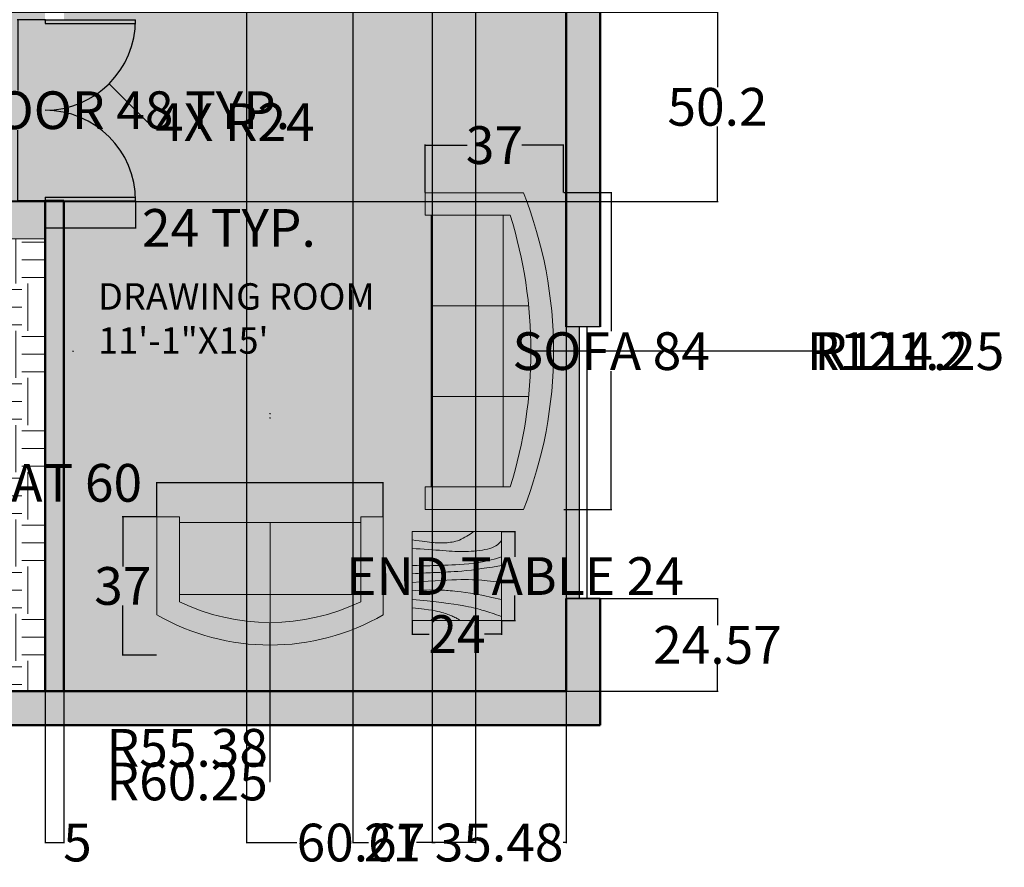
# Model space of a CAD drawing. Units: inches. Extents: x 77 to 548, y 631 to 1307.
# Tile 2 of 4: x 287 to 548, y 631 to 856. Entities that reach past the tile are written whole.
import ezdxf

# ---------------------------------------------------------------- set-up
doc = ezdxf.new("R2010")
doc.units = ezdxf.units.IN
doc.header["$MEASUREMENT"] = 0
for name, color, linetype, lineweight in [('A-ANNO-DIMS', 2, 'Continuous', 18), ('A-AREA-IDEN', 7, 'Continuous', 18), ('A-FLOR-STRS', 7, 'Continuous', 25), ('A-WALL', 7, 'Continuous', 50), ('DOORS', 4, 'Continuous', 25), ('FURNITURE', 34, 'Continuous', 18), ('WINDOW', 6, 'Continuous', 25)]:
    doc.layers.add(name, color=color, linetype=linetype, lineweight=lineweight)
for name, color, linetype, lineweight, true_color in [('A-FLOR-PATT', 254, 'Continuous', 13, 0xd7ebd2), ('A-WALL-PATT', 252, 'Continuous', 13, 0x939598), ('C-PVMT-PATT', 31, 'Continuous', 13, 0xfecc66)]:
    doc.layers.add(name, color=color, linetype=linetype, lineweight=lineweight, true_color=true_color)
doc.styles.get("Standard").update_dxf_attribs({"font": 'arial.ttf'})
doc.dimstyles.get("Standard").update_dxf_attribs({"dimtxt": 10, "dimasz": 0.18, "dimexe": 0.18, "dimexo": 0.0625, "dimgap": 0.09, "dimtad": 0, "dimtih": 1, "dimtoh": 1, "dimdec": 0, "dimzin": 0, "dimdsep": 46, "dimlunit": 3, "dimtxsty": 'Standard', "dimcen": 0.09, "dimadec": 0, "dimazin": 0, "dimtfac": 1, "dimtdec": 0, "dimtofl": 0, "dimtmove": 0, "dimatfit": 3, "dimfxl": 1, "dimtolj": 1, "dimtzin": 0, "dimarcsym": 0})

# ---------------------------------------------------------------- blocks, each defined once
blk = doc.blocks.new('Table - Square Woodgrain 42 x 42 in.')
blk.add_line((0, -42), (42, -42))
for points in [[(0, -4), (1.704, -4.2172), (3.2358, -4.4188), (4.615, -4.604), (5.8615, -4.7721), (6.9951, -4.9224), (8.0357, -5.0541), (9.0031, -5.1667), (9.9171, -5.2594), (10.7951, -5.3316), (11.6445, -5.3836), (12.4702, -5.4157), (13.277, -5.4283), (14.0698, -5.4217), (14.8535, -5.3964), (15.6331, -5.3526), (16.4133, -5.2908), (17.1986, -5.2103), (17.9913, -5.1062), (18.793, -4.9727), (19.6056, -4.8038), (20.4307, -4.5937), (21.2701, -4.3365), (22.1256, -4.0262), (22.9989, -3.6571), (23.888, -3.2272), (24.7756, -2.7516), (25.6408, -2.2491), (26.4624, -1.7387), (27.2195, -1.2395), (27.891, -0.7703), (28.456, -0.3501), (28.8934, 0.002)], [(0, -42), (0, 0), (42, 0), (42, -42)], [(0, -8), (1.8203, -8.1001), (3.6741, -8.2149), (5.5411, -8.3408), (7.4011, -8.4741), (9.2339, -8.6112), (11.0193, -8.7484), (12.7371, -8.8821), (14.3671, -9.0086), (15.8954, -9.1246), (17.3337, -9.2278), (18.6997, -9.3159), (20.0116, -9.387), (21.2871, -9.4389), (22.5442, -9.4696), (23.8008, -9.477), (25.0749, -9.459), (26.3791, -9.4137), (27.7049, -9.3403), (29.0383, -9.2382), (30.3655, -9.1068), (31.6728, -8.9455), (32.9461, -8.7535), (34.1717, -8.5304), (35.3358, -8.2756), (36.4268, -7.9863), (37.443, -7.6521), (38.3849, -7.2603), (39.253, -6.7986), (40.048, -6.2542), (40.7705, -5.6147), (41.421, -4.8674), (42, -4)], [(42, -12), (39.1784, -12.8621), (36.4519, -13.5654), (33.8246, -14.1294), (31.3004, -14.5731), (28.8832, -14.9161), (26.577, -15.1775), (24.3858, -15.3768), (22.3136, -15.5332), (20.3622, -15.6632), (18.5254, -15.7718), (16.7947, -15.8612), (15.1618, -15.9338), (13.6183, -15.9916), (12.1558, -16.0369), (10.7659, -16.0718), (9.4403, -16.0987), (8.1703, -16.1191), (6.9461, -16.1325), (5.7577, -16.1377), (4.595, -16.1335), (3.4479, -16.1188), (2.3064, -16.0924), (1.1604, -16.0532), (0, -16)], [(42, -16), (37.6529, -16.7365), (33.8802, -17.329), (30.6179, -17.7961), (27.8015, -18.1561), (25.3668, -18.4275), (23.2497, -18.6288), (21.3859, -18.7785), (19.7111, -18.8949), (18.1693, -18.9939), (16.7375, -19.0795), (15.401, -19.1534), (14.1449, -19.217), (12.9544, -19.2717), (11.8148, -19.3191), (10.7113, -19.3606), (9.6291, -19.3976), (8.5534, -19.4323), (7.47, -19.4689), (6.3643, -19.5122), (5.222, -19.5672), (4.0288, -19.6386), (2.7703, -19.7313), (1.4321, -19.8501), (0, -20)], [(0, -24), (3.9243, -23.6805), (7.4766, -23.4138), (10.6891, -23.1954), (13.5943, -23.0205), (16.2247, -22.8847), (18.6125, -22.7832), (20.7903, -22.7116), (22.7903, -22.6651), (24.6563, -22.642), (26.4764, -22.6507), (28.35, -22.7024), (30.3766, -22.8084), (32.6555, -22.98), (35.2861, -23.2283), (38.3678, -23.5645), (42, -24)], [(42, -32), (37.392, -31.017), (33.4585, -30.2231), (30.1291, -29.5949), (27.3334, -29.109), (25.0009, -28.742), (23.0612, -28.4707), (21.4439, -28.2716), (20.0786, -28.1215), (18.8998, -28.0002), (17.8609, -27.9014), (16.9206, -27.8219), (16.0371, -27.7588), (15.1691, -27.709), (14.2748, -27.6693), (13.3128, -27.6368), (12.2415, -27.6083), (11.0295, -27.5824), (9.6867, -27.5643), (8.233, -27.5608), (6.6884, -27.5787), (5.0728, -27.6248), (3.4062, -27.7058), (1.7086, -27.8286), (0, -28)], [(0, -32), (5.4026, -32.5358), (9.9494, -33.019), (13.7424, -33.4553), (16.8834, -33.8505), (19.4743, -34.2106), (21.6171, -34.5413), (23.4136, -34.8486), (24.9657, -35.1382), (26.3614, -35.4156), (27.6332, -35.6841), (28.7995, -35.9467), (29.8788, -36.2064), (30.8897, -36.4661), (31.8507, -36.7288), (32.7802, -36.9973), (33.6968, -37.2747), (34.6175, -37.5635), (35.5531, -37.8651), (36.5128, -38.1805), (37.506, -38.5108), (38.5421, -38.8568), (39.6302, -39.2197), (40.7797, -39.6004), (42, -40)], [(0, -36), (3.0098, -36.2857), (5.5354, -36.5643), (7.6368, -36.8359), (9.374, -37.1009), (10.807, -37.3597), (11.9957, -37.6126), (13.0002, -37.8599), (13.8804, -38.102), (14.6874, -38.3393), (15.4365, -38.5729), (16.1338, -38.8041), (16.7858, -39.0341), (17.3987, -39.264), (17.9787, -39.4952), (18.5322, -39.7288), (19.0655, -39.9662), (19.5832, -40.2081), (20.0842, -40.4544), (20.5657, -40.7046), (21.0249, -40.9581), (21.459, -41.2144), (21.8653, -41.4731), (22.2409, -41.7335), (22.5831, -41.9951)]]:
    blk.add_lwpolyline(points)
blk = doc.blocks.new('Sofa - Roundback 7 ft.')
for p, q in [((-12.00002, -32.4421), (-12.00003, -6.5971)), ((11.99997, -32.4421), (11.99998, -6.5971)), ((-36.000027, -34), (-36.000027, -11.4696)), ((35.99998, -34), (35.99998, -11.4696)), ((-35.999844, -13.3819), (35.9998, -13.3819)), ((-36.000027, -32.4421), (35.99998, -32.4421))]:
    blk.add_line(p, q)
for points in [[(-36.000027, -34), (-42.000027, -34), (-42.000027, -8)], [(41.99998, -8), (41.99998, -34), (35.99998, -34)]]:
    blk.add_lwpolyline(points)
for centre, radius, start, end in [((0, -114.25), 114.25, 68.43141, 111.5686), ((-0.00001, -127.1968), 121.1968, 72.72033, 107.2797)]:
    blk.add_arc(centre, radius, start, end)
blk = doc.blocks.new('Sofa - Roundback Loveseat 5 ft.')
for p, q in [((0, -32.44198), (0, -5.99998)), ((-24, -33.99998), (-24, -11.46958)), ((24.00004, -33.99998), (24.00004, -11.46958)), ((-23.9998, -13.38178), (23.99986, -13.38178)), ((-24, -32.44198), (24.00004, -32.44198))]:
    blk.add_line(p, q)
for points in [[(-24, -33.99998), (-30, -33.99998), (-30, -7.99998)], [(30.00004, -7.99998), (30.00004, -33.99998), (24.00004, -33.99998)]]:
    blk.add_lwpolyline(points)
for centre, radius, start, end in [((0, -60.24998), 60.24998, 60.13715, 119.8628), ((0, -61.38438), 55.38444, 64.32083, 115.6792)]:
    blk.add_arc(centre, radius, start, end)
blk = doc.blocks.new('WINDOW-72')
for p, q in [((9, 72), (0, 72)), ((3.5, 72), (3.5, 0)), ((5.5, 72), (5.5, 0)), ((9, 0), (0, 0))]:
    blk.add_line(p, q)
blk = doc.blocks.new('DOOR-DOUBLE-48')
for p, q in [((0, 0), (0, 24)), ((1, 0), (1, 23.98)), ((47, 0), (47, 23.98)), ((48, 0), (48, 24)), ((0, 0), (1, 0)), ((47, 0), (48, 0))]:
    blk.add_line(p, q)
for centre, start, end in [((0, 0), 0, 90), ((48, 0), 90, 180)]:
    blk.add_arc(centre, 24, start, end)
blk = doc.blocks.new('*D26')
at = {"layer": 'A-ANNO-DIMS', "color": 0, "lineweight": -2, "transparency": 16777216}
for p, q in [((293.6, 855.89), (286.28, 855.89)), ((286.46, 855.71), (286.46, 837.15)), ((286.46, 808.07), (286.46, 826.62)), ((293.6, 807.89), (286.28, 807.89))]:
    blk.add_line(p, q, dxfattribs=at)
at = {"layer": 'A-ANNO-DIMS', "color": 0, "transparency": 16777216}
for points in [[(286.43, 855.71), (286.49, 855.71), (286.46, 855.89)], [(286.43, 808.07), (286.49, 808.07), (286.46, 807.89)]]:
    blk.add_solid(points, dxfattribs=at)
at = {"layer": 'Defpoints', "color": 0, "transparency": 16777216}
for p in [(293.66, 855.89), (286.46, 807.89), (293.66, 807.89)]:
    blk.add_point(p, dxfattribs=at)
at = {"layer": 'A-ANNO-DIMS', "color": 0, "transparency": 16777216, "insert": (286.46, 831.89), "char_height": 10, "attachment_point": 5}
blk.add_mtext('\\A1;DOUBLE DOOR 48 TYP.', dxfattribs=at)
blk = doc.blocks.new('*D27')
at = {"layer": 'A-ANNO-DIMS', "color": 0, "lineweight": -2, "transparency": 16777216}
for p, q in [((293.66, 807.83), (293.66, 800.51)), ((317.66, 807.83), (317.66, 800.51)), ((293.84, 800.69), (317.48, 800.69)), ((317.66, 800.69), (317.84, 800.69))]:
    blk.add_line(p, q, dxfattribs=at)
at = {"layer": 'A-ANNO-DIMS', "color": 0, "transparency": 16777216}
for points in [[(293.84, 800.72), (293.84, 800.66), (293.66, 800.69)], [(317.48, 800.72), (317.48, 800.66), (317.66, 800.69)]]:
    blk.add_solid(points, dxfattribs=at)
at = {"layer": 'Defpoints', "color": 0, "transparency": 16777216}
for p in [(293.66, 807.89), (317.66, 807.89), (317.66, 800.69)]:
    blk.add_point(p, dxfattribs=at)
at = {"layer": 'A-ANNO-DIMS', "color": 0, "transparency": 16777216, "insert": (342.36, 800.69), "char_height": 10, "attachment_point": 5}
blk.add_mtext('\\A1;24 TYP.', dxfattribs=at)
blk = doc.blocks.new('*D34')
at = {"layer": 'A-ANNO-DIMS', "color": 0, "lineweight": -2, "transparency": 16777216}
for p, q in [((414.64, 720.24), (418.31, 720.24)), ((418.13, 720.06), (418.13, 713.54)), ((418.13, 696.78), (418.13, 703.31)), ((414.64, 696.6), (418.31, 696.6))]:
    blk.add_line(p, q, dxfattribs=at)
at = {"layer": 'A-ANNO-DIMS', "color": 0, "transparency": 16777216}
for points in [[(418.1, 720.06), (418.16, 720.06), (418.13, 720.24)], [(418.1, 696.78), (418.16, 696.78), (418.13, 696.6)]]:
    blk.add_solid(points, dxfattribs=at)
at = {"layer": 'Defpoints', "color": 0, "transparency": 16777216}
for p in [(414.58, 720.24), (418.13, 720.24), (414.58, 696.6)]:
    blk.add_point(p, dxfattribs=at)
at = {"layer": 'A-ANNO-DIMS', "color": 0, "transparency": 16777216, "insert": (418.13, 708.42), "char_height": 10, "attachment_point": 5}
blk.add_mtext('\\A1;END TABLE 24', dxfattribs=at)
blk = doc.blocks.new('*D35')
at = {"layer": 'A-ANNO-DIMS', "color": 0, "lineweight": -2, "transparency": 16777216}
for p, q in [((390.94, 696.54), (390.94, 692.87)), ((414.58, 696.54), (414.58, 692.87)), ((391.12, 693.05), (395.44, 693.05)), ((414.4, 693.05), (410.08, 693.05))]:
    blk.add_line(p, q, dxfattribs=at)
at = {"layer": 'A-ANNO-DIMS', "color": 0, "transparency": 16777216}
for points in [[(391.12, 693.08), (391.12, 693.02), (390.94, 693.05)], [(414.4, 693.08), (414.4, 693.02), (414.58, 693.05)]]:
    blk.add_solid(points, dxfattribs=at)
at = {"layer": 'Defpoints', "color": 0, "transparency": 16777216}
for p in [(390.94, 696.6), (414.58, 696.6), (414.58, 693.05)]:
    blk.add_point(p, dxfattribs=at)
at = {"layer": 'A-ANNO-DIMS', "color": 0, "transparency": 16777216, "insert": (402.76, 693.05), "char_height": 10, "attachment_point": 5}
blk.add_mtext('\\A1;24', dxfattribs=at)
blk = doc.blocks.new('*D38')
at = {"layer": 'A-ANNO-DIMS', "color": 0, "lineweight": -2, "transparency": 16777216}
for p, q in [((431.08, 810.04), (443.79, 810.04)), ((443.61, 809.86), (443.61, 773.3)), ((443.61, 726.22), (443.61, 762.77)), ((431.08, 726.04), (443.79, 726.04))]:
    blk.add_line(p, q, dxfattribs=at)
at = {"layer": 'A-ANNO-DIMS', "color": 0, "transparency": 16777216}
for points in [[(443.58, 809.86), (443.64, 809.86), (443.61, 810.04)], [(443.58, 726.22), (443.64, 726.22), (443.61, 726.04)]]:
    blk.add_solid(points, dxfattribs=at)
at = {"layer": 'Defpoints', "color": 0, "transparency": 16777216}
for p in [(431.01, 810.04), (431.01, 726.04), (443.61, 726.04)]:
    blk.add_point(p, dxfattribs=at)
at = {"layer": 'A-ANNO-DIMS', "color": 0, "transparency": 16777216, "insert": (443.61, 768.04), "char_height": 10, "attachment_point": 5}
blk.add_mtext('\\A1;SOFA 84', dxfattribs=at)
blk = doc.blocks.new('*D39')
at = {"layer": 'A-ANNO-DIMS', "color": 0, "lineweight": -2, "transparency": 16777216}
for p, q in [((394.35, 810.1), (394.35, 822.82)), ((394.53, 822.64), (405.43, 822.64)), ((430.83, 822.64), (419.93, 822.64)), ((431.01, 810.1), (431.01, 822.82))]:
    blk.add_line(p, q, dxfattribs=at)
at = {"layer": 'A-ANNO-DIMS', "color": 0, "transparency": 16777216}
for points in [[(394.53, 822.67), (394.53, 822.61), (394.35, 822.64)], [(430.83, 822.67), (430.83, 822.61), (431.01, 822.64)]]:
    blk.add_solid(points, dxfattribs=at)
at = {"layer": 'Defpoints', "color": 0, "transparency": 16777216}
for p in [(431.01, 822.64), (394.35, 810.04), (431.01, 810.04)]:
    blk.add_point(p, dxfattribs=at)
at = {"layer": 'A-ANNO-DIMS', "color": 0, "transparency": 16777216, "insert": (412.68, 822.64), "char_height": 10, "attachment_point": 5}
blk.add_mtext('\\A1;37', dxfattribs=at)
blk = doc.blocks.new('*D40')
at = {"layer": 'A-ANNO-DIMS', "color": 0, "lineweight": -2, "transparency": 16777216}
for p, q in [((323.26, 733.13), (323.08, 733.13)), ((323.26, 724.2), (323.26, 733.31)), ((383.08, 733.13), (323.44, 733.13)), ((383.26, 724.2), (383.26, 733.31))]:
    blk.add_line(p, q, dxfattribs=at)
at = {"layer": 'A-ANNO-DIMS', "color": 0, "transparency": 16777216}
for points in [[(323.44, 733.16), (323.44, 733.1), (323.26, 733.13)], [(383.08, 733.16), (383.08, 733.1), (383.26, 733.13)]]:
    blk.add_solid(points, dxfattribs=at)
at = {"layer": 'Defpoints', "color": 0, "transparency": 16777216}
for p in [(323.26, 733.13), (323.26, 724.13), (383.26, 724.13)]:
    blk.add_point(p, dxfattribs=at)
at = {"layer": 'A-ANNO-DIMS', "color": 0, "transparency": 16777216, "insert": (277.25, 733.13), "char_height": 10, "attachment_point": 5}
blk.add_mtext('\\A1;LOVESEAT 60', dxfattribs=at)
blk = doc.blocks.new('*D41')
at = {"layer": 'A-ANNO-DIMS', "color": 0, "lineweight": -2, "transparency": 16777216}
for p, q in [((323.2, 724.13), (314.08, 724.13)), ((314.26, 723.95), (314.26, 711)), ((314.26, 687.65), (314.26, 700.6)), ((323.2, 687.47), (314.08, 687.47))]:
    blk.add_line(p, q, dxfattribs=at)
at = {"layer": 'A-ANNO-DIMS', "color": 0, "transparency": 16777216}
for points in [[(314.23, 723.95), (314.29, 723.95), (314.26, 724.13)], [(314.23, 687.65), (314.29, 687.65), (314.26, 687.47)]]:
    blk.add_solid(points, dxfattribs=at)
at = {"layer": 'Defpoints', "color": 0, "transparency": 16777216}
for p in [(323.26, 724.13), (314.26, 687.47), (323.26, 687.47)]:
    blk.add_point(p, dxfattribs=at)
at = {"layer": 'A-ANNO-DIMS', "color": 0, "transparency": 16777216, "insert": (314.26, 705.8), "char_height": 10, "attachment_point": 5}
blk.add_mtext('\\A1;37', dxfattribs=at)
blk = doc.blocks.new('*D45')
at = {"layer": 'A-ANNO-DIMS', "color": 0, "lineweight": -2, "transparency": 16777216}
for p, q in [((293.66, 677.83), (293.66, 637.61)), ((298.66, 677.83), (298.66, 637.61)), ((293.84, 637.79), (298.48, 637.79)), ((298.66, 637.79), (298.84, 637.79))]:
    blk.add_line(p, q, dxfattribs=at)
at = {"layer": 'A-ANNO-DIMS', "color": 0, "transparency": 16777216}
for points in [[(293.84, 637.82), (293.84, 637.76), (293.66, 637.79)], [(298.48, 637.82), (298.48, 637.76), (298.66, 637.79)]]:
    blk.add_solid(points, dxfattribs=at)
at = {"layer": 'Defpoints', "color": 0, "transparency": 16777216}
for p in [(293.66, 677.89), (298.66, 677.89), (298.66, 637.79)]:
    blk.add_point(p, dxfattribs=at)
at = {"layer": 'A-ANNO-DIMS', "color": 0, "transparency": 16777216, "insert": (302.25, 637.79), "char_height": 10, "attachment_point": 5}
blk.add_mtext('\\A1;5', dxfattribs=at)
blk = doc.blocks.new('*D46')
at = {"layer": 'A-ANNO-DIMS', "color": 0, "lineweight": -2, "transparency": 16777216}
for p, q in [((431.73, 702.46), (471.94, 702.46)), ((471.76, 702.28), (471.76, 695.37)), ((471.76, 678.07), (471.76, 684.98)), ((431.73, 677.89), (471.94, 677.89))]:
    blk.add_line(p, q, dxfattribs=at)
at = {"layer": 'A-ANNO-DIMS', "color": 0, "transparency": 16777216}
for points in [[(471.73, 702.28), (471.79, 702.28), (471.76, 702.46)], [(471.73, 678.07), (471.79, 678.07), (471.76, 677.89)]]:
    blk.add_solid(points, dxfattribs=at)
at = {"layer": 'Defpoints', "color": 0, "transparency": 16777216}
for p in [(431.66, 702.46), (471.76, 702.46), (431.66, 677.89)]:
    blk.add_point(p, dxfattribs=at)
at = {"layer": 'A-ANNO-DIMS', "color": 0, "transparency": 16777216, "insert": (471.76, 690.17), "char_height": 10, "attachment_point": 5}
blk.add_mtext('\\A1;24.57', dxfattribs=at)
blk = doc.blocks.new('*D57')
at = {"layer": 'A-ANNO-DIMS', "color": 0, "lineweight": -2, "transparency": 16777216}
for p, q in [((346.99, 920.83), (346.99, 637.61)), ((407.66, 920.83), (407.66, 637.61)), ((347.17, 637.79), (360.34, 637.79)), ((407.48, 637.79), (394.32, 637.79))]:
    blk.add_line(p, q, dxfattribs=at)
at = {"layer": 'A-ANNO-DIMS', "color": 0, "transparency": 16777216}
for points in [[(347.17, 637.82), (347.17, 637.76), (346.99, 637.79)], [(407.48, 637.82), (407.48, 637.76), (407.66, 637.79)]]:
    blk.add_solid(points, dxfattribs=at)
at = {"layer": 'Defpoints', "color": 0, "transparency": 16777216}
for p in [(346.99, 920.89), (407.66, 920.89), (407.66, 637.79)]:
    blk.add_point(p, dxfattribs=at)
at = {"layer": 'A-ANNO-DIMS', "color": 0, "transparency": 16777216, "insert": (377.33, 637.79), "char_height": 10, "attachment_point": 5}
blk.add_mtext('\\A1;60.67', dxfattribs=at)
blk = doc.blocks.new('*D58')
at = {"layer": 'A-ANNO-DIMS', "color": 0, "lineweight": -2, "transparency": 16777216}
for p, q in [((375.18, 949.83), (375.18, 637.61)), ((396.18, 949.83), (396.18, 637.61)), ((375.36, 637.79), (379.31, 637.79)), ((396, 637.79), (392.05, 637.79))]:
    blk.add_line(p, q, dxfattribs=at)
at = {"layer": 'A-ANNO-DIMS', "color": 0, "transparency": 16777216}
for points in [[(375.36, 637.82), (375.36, 637.76), (375.18, 637.79)], [(396, 637.82), (396, 637.76), (396.18, 637.79)]]:
    blk.add_solid(points, dxfattribs=at)
at = {"layer": 'Defpoints', "color": 0, "transparency": 16777216}
for p in [(375.18, 949.89), (396.18, 949.89), (396.18, 637.79)]:
    blk.add_point(p, dxfattribs=at)
at = {"layer": 'A-ANNO-DIMS', "color": 0, "transparency": 16777216, "insert": (385.68, 637.79), "char_height": 10, "attachment_point": 5}
blk.add_mtext('\\A1;21', dxfattribs=at)
blk = doc.blocks.new('*D60')
at = {"layer": 'A-ANNO-DIMS', "color": 0, "lineweight": -2, "transparency": 16777216}
for p, q in [((396.18, 949.83), (396.18, 637.61)), ((431.66, 949.83), (431.66, 637.61)), ((396.36, 637.79), (396.95, 637.79)), ((431.48, 637.79), (430.89, 637.79))]:
    blk.add_line(p, q, dxfattribs=at)
at = {"layer": 'A-ANNO-DIMS', "color": 0, "transparency": 16777216}
for points in [[(396.36, 637.82), (396.36, 637.76), (396.18, 637.79)], [(431.48, 637.82), (431.48, 637.76), (431.66, 637.79)]]:
    blk.add_solid(points, dxfattribs=at)
at = {"layer": 'Defpoints', "color": 0, "transparency": 16777216}
for p in [(396.18, 949.89), (431.66, 949.89), (431.66, 637.79)]:
    blk.add_point(p, dxfattribs=at)
at = {"layer": 'A-ANNO-DIMS', "color": 0, "transparency": 16777216, "insert": (413.92, 637.79), "char_height": 10, "attachment_point": 5}
blk.add_mtext('\\A1;35.48', dxfattribs=at)
blk = doc.blocks.new('*D62')
at = {"layer": 'A-ANNO-DIMS', "color": 0, "lineweight": -2, "transparency": 16777216}
for p, q in [((243.73, 857.89), (471.94, 857.89)), ((471.76, 857.71), (471.76, 837.98)), ((471.76, 807.86), (471.76, 827.59)), ((243.73, 807.68), (471.94, 807.68))]:
    blk.add_line(p, q, dxfattribs=at)
at = {"layer": 'A-ANNO-DIMS', "color": 0, "transparency": 16777216}
for points in [[(471.73, 857.71), (471.79, 857.71), (471.76, 857.89)], [(471.73, 807.86), (471.79, 807.86), (471.76, 807.68)]]:
    blk.add_solid(points, dxfattribs=at)
at = {"layer": 'Defpoints', "color": 0, "transparency": 16777216}
for p in [(243.66, 857.89), (471.76, 857.89), (243.66, 807.68)]:
    blk.add_point(p, dxfattribs=at)
at = {"layer": 'A-ANNO-DIMS', "color": 0, "transparency": 16777216, "insert": (471.76, 832.79), "char_height": 10, "attachment_point": 5}
blk.add_mtext('\\A1;50.2', dxfattribs=at)
blk = doc.blocks.new('*D64')
at = {"layer": 'A-ANNO-DIMS', "color": 0, "lineweight": -2, "transparency": 16777216}
for p, q in [((301.06, 768.04), (301.24, 768.04)), ((301.15, 767.95), (301.15, 768.13)), ((495.07, 768.04), (422.53, 768.04))]:
    blk.add_line(p, q, dxfattribs=at)
at = {"layer": 'A-ANNO-DIMS', "color": 0, "transparency": 16777216}
blk.add_solid([(422.53, 768.07), (422.53, 768.01), (422.35, 768.04)], dxfattribs=at)
at = {"layer": 'Defpoints', "color": 0, "transparency": 16777216}
for p in [(301.15, 768.04), (422.35, 768.04)]:
    blk.add_point(p, dxfattribs=at)
at = {"layer": 'A-ANNO-DIMS', "color": 0, "transparency": 16777216, "insert": (516.76, 768.04), "char_height": 10, "attachment_point": 5}
blk.add_mtext('\\A1;R121.2', dxfattribs=at)
blk = doc.blocks.new('*D65')
at = {"layer": 'A-ANNO-DIMS', "color": 0, "lineweight": -2, "transparency": 16777216}
for p, q in [((314.01, 768.04), (314.19, 768.04)), ((314.1, 767.95), (314.1, 768.13)), ((496.9, 768.04), (428.53, 768.04))]:
    blk.add_line(p, q, dxfattribs=at)
at = {"layer": 'A-ANNO-DIMS', "color": 0, "transparency": 16777216}
blk.add_solid([(428.53, 768.07), (428.53, 768.01), (428.35, 768.04)], dxfattribs=at)
at = {"layer": 'Defpoints', "color": 0, "transparency": 16777216}
for p in [(314.1, 768.04), (428.35, 768.04)]:
    blk.add_point(p, dxfattribs=at)
at = {"layer": 'A-ANNO-DIMS', "color": 0, "transparency": 16777216, "insert": (522.57, 768.04), "char_height": 10, "attachment_point": 5}
blk.add_mtext('\\A1;R114.25', dxfattribs=at)
blk = doc.blocks.new('*D66')
at = {"layer": 'A-ANNO-DIMS', "color": 0, "lineweight": -2, "transparency": 16777216}
for p, q in [((353.17, 750.38), (353.35, 750.38)), ((353.26, 750.29), (353.26, 750.47)), ((353.26, 653.98), (353.26, 689.95)), ((353.08, 653.98), (353.26, 653.98))]:
    blk.add_line(p, q, dxfattribs=at)
at = {"layer": 'A-ANNO-DIMS', "color": 0, "transparency": 16777216}
blk.add_solid([(353.23, 689.95), (353.29, 689.95), (353.26, 690.13)], dxfattribs=at)
at = {"layer": 'Defpoints', "color": 0, "transparency": 16777216}
for p in [(353.26, 750.38), (353.26, 690.13)]:
    blk.add_point(p, dxfattribs=at)
at = {"layer": 'A-ANNO-DIMS', "color": 0, "transparency": 16777216, "insert": (331.3, 653.98), "char_height": 10, "attachment_point": 5}
blk.add_mtext('\\A1;R60.25', dxfattribs=at)
blk = doc.blocks.new('*D67')
at = {"layer": 'A-ANNO-DIMS', "color": 0, "lineweight": -2, "transparency": 16777216}
for p, q in [((353.17, 751.52), (353.35, 751.52)), ((353.26, 751.43), (353.26, 751.61)), ((353.26, 662.9), (353.26, 695.95)), ((353.08, 662.9), (353.26, 662.9))]:
    blk.add_line(p, q, dxfattribs=at)
at = {"layer": 'A-ANNO-DIMS', "color": 0, "transparency": 16777216}
blk.add_solid([(353.23, 695.95), (353.29, 695.95), (353.26, 696.13)], dxfattribs=at)
at = {"layer": 'Defpoints', "color": 0, "transparency": 16777216}
for p in [(353.26, 751.52), (353.26, 696.13)]:
    blk.add_point(p, dxfattribs=at)
at = {"layer": 'A-ANNO-DIMS', "color": 0, "transparency": 16777216, "insert": (331.33, 662.9), "char_height": 10, "attachment_point": 5}
blk.add_mtext('\\A1;R55.38', dxfattribs=at)
blk = doc.blocks.new('*D68')
at = {"layer": 'A-ANNO-DIMS', "color": 0, "lineweight": -2, "transparency": 16777216}
for p, q in [((293.57, 855.89), (293.75, 855.89)), ((293.66, 855.8), (293.66, 855.98)), ((320.82, 828.74), (310.76, 838.79)), ((321, 828.74), (320.82, 828.74))]:
    blk.add_line(p, q, dxfattribs=at)
at = {"layer": 'A-ANNO-DIMS', "color": 0, "transparency": 16777216}
blk.add_solid([(310.78, 838.81), (310.74, 838.77), (310.63, 838.92)], dxfattribs=at)
at = {"layer": 'Defpoints', "color": 0, "transparency": 16777216}
for p in [(293.66, 855.89), (310.63, 838.92)]:
    blk.add_point(p, dxfattribs=at)
at = {"layer": 'A-ANNO-DIMS', "color": 0, "transparency": 16777216, "insert": (343.96, 828.74), "char_height": 10, "attachment_point": 5}
blk.add_mtext('\\A1;4X R24', dxfattribs=at)

msp = doc.modelspace()

# ---------------------------------------------------------------- hatches: boundary and pattern name
at = {"layer": 'A-FLOR-PATT'}
h = msp.add_hatch(color=256, dxfattribs=at)
h.dxf.hatch_style = 1
h.paths.add_polyline_path([(293.663, 1206.888), (291.663, 1206.888), (291.663, 1211.888), (293.663, 1211.888), (293.663, 1259.888), (149.663, 1259.888), (149.663, 1211.888), (257.663, 1211.888), (257.663, 1206.888), (245.663, 1206.888), (245.663, 1204.888), (245.663, 1174.888), (245.663, 1153.888), (149.663, 1153.888), (149.663, 1047.888), (255.663, 1047.888), (255.663, 1042.888), (149.663, 1042.888), (149.663, 988.888), (146.163, 988.888), (146.163, 916.888), (149.663, 916.888), (149.663, 862.888), (243.663, 862.888), (243.663, 857.888), (243.663, 807.683), (293.663, 807.888), (298.663, 807.888), (298.663, 677.888), (431.663, 677.888), (431.663, 702.459), (435.163, 702.459), (435.163, 774.459), (431.663, 774.459), (431.663, 857.888), (330.663, 857.888), (330.663, 862.888), (325.663, 944.888), (325.663, 949.888), (346.663, 949.888), (346.663, 965.888), (346.663, 995.888), (346.663, 997.888), (293.663, 997.888), (293.663, 1002.888), (293.663, 1004.888), (298.663, 1004.888), (298.663, 1002.888), (431.663, 1002.888), (431.663, 1095.888), (431.663, 1100.888), (431.663, 1147.888), (342.663, 1147.888), (342.663, 1174.888), (342.663, 1204.888), (342.663, 1206.888), (334.663, 1206.888), (334.663, 1211.888), (431.663, 1211.888), (431.663, 1259.888), (298.663, 1259.888), (298.663, 1211.888), (300.663, 1211.888), (300.663, 1206.888), (298.663, 1206.888), (298.663, 1042.888), (298.663, 1040.888), (293.663, 1040.888), (291.663, 1040.888), (291.663, 1047.888), (293.663, 1047.888)])
h.paths.add_polyline_path([(291.663, 862.888), (293.663, 862.888), (298.663, 862.888), (300.663, 862.888), (300.663, 857.888), (298.663, 857.888), (298.663, 855.888), (293.663, 855.888), (293.663, 857.888), (291.663, 857.888)], flags=16)
h.paths.add_polyline_path([(407.663, 920.888), (346.988, 920.888), (346.988, 944.888), (325.663, 944.888), (330.663, 862.888), (407.663, 862.888)], flags=17)
h.paths.add_polyline_path([(435.163, 988.679), (431.663, 988.679), (431.663, 997.888), (351.663, 997.888), (351.663, 995.888), (346.663, 995.888), (346.663, 965.888), (351.663, 965.888), (351.663, 949.888), (375.18, 949.888), (375.18, 957.888), (381.68, 957.888), (379.68, 963.887, -0.7025712), (385.68, 977.887, -0.7025621), (391.68, 963.888), (389.68, 957.888), (392.68, 957.888), (392.68, 959.388), (395.68, 959.388), (395.68, 957.888), (396.18, 957.888), (396.18, 949.888), (431.663, 949.888), (431.663, 964.679), (435.163, 964.679)])
h.paths.add_polyline_path([(431.663, 1206.888), (347.663, 1206.888), (347.663, 1204.888), (342.663, 1204.888), (342.663, 1174.888), (347.663, 1174.888), (347.663, 1167.048), (372.327, 1167.048), (372.327, 1152.888), (374.776, 1152.888), (374.776, 1160.888), (381.276, 1160.888), (379.276, 1166.887, -0.7025712), (385.276, 1180.887, -0.7025621), (391.276, 1166.888), (389.276, 1160.888), (392.276, 1160.888), (392.276, 1162.388), (395.276, 1162.388), (395.276, 1160.888), (395.776, 1160.888), (395.776, 1152.888), (431.663, 1152.888), (431.663, 1170.888), (435.163, 1170.888), (435.163, 1194.888), (431.663, 1194.888)])
h.paths.add_polyline_path([(245.663, 1204.888), (240.663, 1204.888), (240.663, 1206.888), (149.663, 1206.888), (149.663, 1194.888), (146.163, 1194.888), (146.163, 1170.888), (149.663, 1170.888), (149.663, 1158.888), (188.741, 1158.888), (188.741, 1166.888), (195.241, 1166.888), (193.241, 1172.887, -0.7025712), (199.241, 1186.887, -0.7025621), (205.241, 1172.888), (203.241, 1166.888), (206.241, 1166.888), (206.241, 1168.388), (209.241, 1168.388), (209.241, 1166.888), (209.741, 1166.888), (209.741, 1158.888), (215.999, 1158.888), (215.999, 1173.048), (240.663, 1173.048), (240.663, 1174.888), (245.663, 1174.888)], flags=17)
at = {"layer": 'A-WALL-PATT'}
h = msp.add_hatch(color=256, dxfattribs=at)
h.dxf.hatch_style = 1
h.paths.add_polyline_path([(149.663, 1042.888), (149.663, 1170.888), (140.663, 1170.888), (140.663, 988.888), (149.663, 988.888)])
h.paths.add_polyline_path([(149.663, 1259.888), (431.663, 1259.888), (431.663, 1194.888), (440.663, 1194.888), (440.663, 1268.888), (140.663, 1268.888), (140.663, 1194.888), (149.663, 1194.888), (149.663, 1206.888)])
h.paths.add_polyline_path([(298.663, 1259.888), (293.663, 1259.888), (293.663, 1211.888), (291.663, 1211.888), (291.663, 1206.888), (293.663, 1206.888), (293.663, 1047.888), (291.663, 1047.888), (291.663, 1040.888), (293.663, 1040.888), (298.663, 1040.888), (298.663, 1095.888), (298.663, 1206.888), (300.663, 1206.888), (300.663, 1211.888), (298.663, 1211.888)])
h.paths.add_polyline_path([(257.663, 1211.888), (149.663, 1211.888), (149.663, 1206.888), (240.663, 1206.888), (240.663, 1204.888), (241.135, 1204.888), (245.663, 1204.888), (245.663, 1206.888), (257.663, 1206.888)], flags=17)
h.paths.add_polyline_path([(431.663, 1211.888), (334.663, 1211.888), (334.663, 1206.888), (342.663, 1206.888), (342.663, 1204.888), (347.191, 1204.888), (347.663, 1204.888), (347.663, 1206.888), (431.663, 1206.888)], flags=17)
h.paths.add_polyline_path([(440.663, 1170.888), (431.663, 1170.888), (431.663, 1100.888), (431.663, 1047.888), (431.663, 988.679), (440.663, 988.679)])
h.paths.add_polyline_path([(431.663, 1002.888), (298.663, 1002.888), (298.663, 1004.888), (293.663, 1004.888), (293.663, 1002.888), (293.663, 997.888), (346.663, 997.888), (346.663, 995.888), (351.663, 995.888), (351.663, 997.888), (431.663, 997.888)])
h.paths.add_polyline_path([(440.663, 964.679), (431.663, 964.679), (431.663, 949.888), (351.663, 949.888), (351.663, 965.888), (346.663, 965.888), (346.663, 949.888), (325.663, 949.888), (325.663, 944.888), (431.663, 944.888), (431.663, 915.45), (440.663, 915.45)])
h.paths.add_polyline_path([(440.663, 891.45), (431.663, 891.45), (431.663, 862.888), (330.663, 862.888), (330.663, 857.888), (431.663, 857.888), (431.663, 774.459), (440.663, 774.459)], flags=17)
h.paths.add_polyline_path([(440.663, 702.459), (431.663, 702.459), (431.663, 677.888), (149.663, 677.888), (149.663, 916.888), (140.663, 916.888), (140.663, 668.888), (440.663, 668.888)])
h.paths.add_polyline_path([(293.663, 807.888), (243.663, 807.683), (243.663, 857.888), (233.663, 857.888), (233.663, 807.683), (233.663, 797.642), (243.704, 797.683), (293.663, 797.887)], flags=17)
h.paths.add_polyline_path([(243.663, 862.888), (149.663, 862.888), (149.663, 857.888), (243.663, 857.888)], flags=17)
h = msp.add_hatch(color=256, dxfattribs=at)
h.dxf.hatch_style = 1
h.paths.add_polyline_path([(298.663, 807.888), (293.663, 807.888), (293.663, 677.888), (298.663, 677.888)])
h.paths.add_polyline_path([(255.663, 1047.888), (149.663, 1047.888), (149.663, 1042.888), (255.663, 1042.888)])
h.paths.add_polyline_path([(245.663, 1174.888), (240.663, 1174.888), (240.663, 1158.888), (215.999, 1158.888), (149.663, 1158.888), (149.663, 1153.888), (245.663, 1153.888)])
h.paths.add_polyline_path([(347.663, 1167.048), (347.663, 1174.888), (342.663, 1174.888), (342.663, 1147.888), (431.663, 1147.888), (431.663, 1152.888), (347.663, 1152.888)])
at = {"layer": 'C-PVMT-PATT'}
h = msp.add_hatch(dxfattribs=at)
h.set_pattern_fill('EARTH', color=256, scale=50)
h.paths.add_polyline_path([(293.663, 797.887), (243.704, 797.683), (233.663, 797.642), (233.663, 807.683), (233.663, 857.888), (149.663, 857.888), (149.663, 677.888), (293.663, 677.888)])

# ---------------------------------------------------------------- linework, layer by layer
at = {"layer": 'A-FLOR-STRS'}
for p, q in [((243.663, 807.683), (293.663, 807.888)), ((243.704, 797.683), (293.704, 797.888))]:
    msp.add_line(p, q, dxfattribs=at)
at = {"layer": 'A-WALL'}
for p, q in [((440.663, 774.459), (440.663, 891.45)), ((431.663, 774.459), (431.663, 857.888)), ((293.663, 807.888), (293.663, 677.888)), ((293.663, 677.888), (293.663, 807.888)), ((293.663, 807.888), (298.663, 807.888)), ((293.663, 807.888), (298.663, 807.888)), ((298.663, 807.888), (298.663, 677.888)), ((298.663, 677.888), (298.663, 807.888)), ((431.663, 677.888), (431.663, 702.459)), ((440.663, 668.888), (440.663, 702.459)), ((149.663, 677.888), (431.663, 677.888)), ((140.663, 668.888), (440.663, 668.888))]:
    msp.add_line(p, q, dxfattribs=at)

# ---------------------------------------------------------------- block references
at = {"layer": 'DOORS', "rotation": 270.0000000000005}
msp.add_blockref('DOOR-DOUBLE-48', (293.663, 855.888), dxfattribs=at)
at = {"layer": 'FURNITURE'}
for name, p, rotation in [('Sofa - Roundback 7 ft.', (428.348, 768.036), 270), ('Sofa - Roundback Loveseat 5 ft.', (353.263, 690.133), 180)]:
    msp.add_blockref(name, p, dxfattribs=dict(at, rotation=rotation))
at = {"layer": 'FURNITURE', "xscale": 0.5629009411423532, "yscale": 0.5629009411423532, "zscale": 0.5629009411423532}
msp.add_blockref('Table - Square Woodgrain 42 x 42 in.', (390.938, 720.242), dxfattribs=at)
at = {"layer": 'WINDOW'}
msp.add_blockref('WINDOW-72', (431.663, 702.459), dxfattribs=at)

# ---------------------------------------------------------------- texts
at = {"layer": 'A-AREA-IDEN', "insert": (307.738, 786.034), "char_height": 5, "attachment_point": 1}
msp.add_mtext_dynamic_manual_height_columns('{\\H1.4x;DRAWING ROOM\\P11\'-1"X15\'}', width=99.94444, gutter_width=1, heights=[50.869], dxfattribs=at)

# ---------------------------------------------------------------- dimensions: what is measured, and where the dimension line sits
at = {"layer": 'A-ANNO-DIMS'}
for base, p1, p2, override, picture, middle in [((396.18, 637.788), (375.18, 949.888), (396.18, 949.888), {"dimdec": 0, "dimlfac": 1, "dimrnd": 0, "dimzin": 0, "dimdsep": 46, "dimlunit": 2}, '*D58', (385.68, 637.788)), ((431.663, 637.788), (396.18, 949.888), (431.663, 949.888), {"dimdec": 2, "dimlfac": 1, "dimrnd": 0, "dimzin": 0, "dimdsep": 46, "dimlunit": 2}, '*D60', (413.922, 637.788)), ((407.663, 637.7875), (346.9885, 920.8875), (407.663, 920.8875), {"dimdec": 2, "dimlfac": 1, "dimrnd": 0, "dimzin": 0, "dimdsep": 46, "dimlunit": 2}, '*D57', (377.3257, 637.7875)), ((431.015, 822.636), (394.348, 810.036), (431.015, 810.036), {"dimdec": 0, "dimlfac": 1, "dimrnd": 0, "dimzin": 0, "dimdsep": 46, "dimlunit": 2}, '*D39', (412.681, 822.636)), ((414.579, 693.053), (390.938, 696.6), (414.579, 696.6), {"dimdec": 0, "dimlfac": 1, "dimrnd": 0, "dimzin": 0, "dimdsep": 46, "dimlunit": 2}, '*D35', (402.759, 693.053)), ((298.663, 637.788), (293.663, 677.888), (298.663, 677.888), {"dimdec": 0, "dimlfac": 1, "dimrnd": 0, "dimzin": 0, "dimdsep": 46, "dimlunit": 2}, '*D45', (302.248, 637.788))]:
    dim = msp.add_linear_dim(base=base, p1=p1, p2=p2, dimstyle='Standard', override=override, dxfattribs=at)
    dim.commit()
    dim.dimension.update_dxf_attribs({"geometry": picture, "text_midpoint": middle})
for base, p1, p2, angle, text, picture, middle in [((286.463, 807.888), (293.663, 855.888), (293.663, 807.888), 270, 'DOUBLE DOOR <> TYP.', '*D26', (286.463, 831.888)), ((317.663, 800.688), (293.663, 807.888), (317.663, 807.888), 0, '<> TYP.', '*D27', (342.357, 800.688)), ((443.615, 726.036), (431.015, 810.036), (431.015, 726.036), 270, 'SOFA <>', '*D38', (443.615, 768.036)), ((323.263, 733.133), (383.263, 724.133), (323.263, 724.133), 180, 'LOVESEAT <>', '*D40', (277.25, 733.133)), ((418.126, 720.243), (414.579, 696.6), (414.579, 720.243), 90, 'END TABLE <>', '*D34', (418.126, 708.421))]:
    dim = msp.add_linear_dim(base=base, p1=p1, p2=p2, angle=angle, text=text, dimstyle='Standard', override={"dimdec": 0, "dimlfac": 1, "dimrnd": 0, "dimzin": 0, "dimdsep": 46, "dimlunit": 2}, dxfattribs=at)
    dim.commit()
    dim.dimension.update_dxf_attribs({"geometry": picture, "text_midpoint": middle})
for base, p1, p2, angle, override, picture, middle in [((471.763, 857.888), (243.663, 807.683), (243.663, 857.888), 90, {"dimdec": 1, "dimlfac": 1, "dimrnd": 0, "dimzin": 0, "dimdsep": 46, "dimlunit": 2}, '*D62', (471.763, 832.785)), ((314.263, 687.466), (323.263, 724.133), (323.263, 687.466), 270, {"dimdec": 0, "dimlfac": 1, "dimrnd": 0, "dimzin": 0, "dimdsep": 46, "dimlunit": 2}, '*D41', (314.263, 705.799)), ((471.763, 702.459), (431.663, 677.888), (431.663, 702.459), 90, {"dimdec": 2, "dimlfac": 1, "dimrnd": 0, "dimzin": 0, "dimdsep": 46, "dimlunit": 2}, '*D46', (471.763, 690.173))]:
    dim = msp.add_linear_dim(base=base, p1=p1, p2=p2, angle=angle, dimstyle='Standard', override=override, dxfattribs=at)
    dim.commit()
    dim.dimension.update_dxf_attribs({"geometry": picture, "text_midpoint": middle})
dim = msp.add_radius_dim(center=(293.663, 855.888), mpoint=(310.634, 838.917), text='4X <>', dimstyle='Standard', override={"dimdec": 0, "dimlfac": 1, "dimrnd": 0, "dimzin": 0, "dimdsep": 46, "dimlunit": 2}, dxfattribs=at)
dim.commit()
dim.dimension.update_dxf_attribs({"geometry": '*D68', "text_midpoint": (343.958, 828.735), "dimtype": 164})
for center, mpoint, override, picture, middle in [((301.151, 768.036), (422.348, 768.036), {"dimdec": 1, "dimlfac": 1, "dimrnd": 0, "dimzin": 0, "dimdsep": 46, "dimlunit": 2}, '*D64', (495.066, 768.036)), ((314.098, 768.036), (428.348, 768.036), {"dimdec": 2, "dimlfac": 1, "dimrnd": 0, "dimzin": 0, "dimdsep": 46, "dimlunit": 2}, '*D65', (496.898, 768.036)), ((353.263, 751.517), (353.263, 696.133), {"dimdec": 2, "dimlfac": 1, "dimrnd": 0, "dimzin": 0, "dimdsep": 46, "dimlunit": 2}, '*D67', (331.325, 662.902)), ((353.263, 750.383), (353.263, 690.133), {"dimdec": 2, "dimlfac": 1, "dimrnd": 0, "dimzin": 0, "dimdsep": 46, "dimlunit": 2}, '*D66', (331.298, 653.983))]:
    dim = msp.add_radius_dim(center=center, mpoint=mpoint, dimstyle='Standard', override=override, dxfattribs=at)
    dim.commit()
    dim.dimension.update_dxf_attribs({"geometry": picture, "text_midpoint": middle, "dimtype": 164})

doc.saveas('drawing.dxf')
